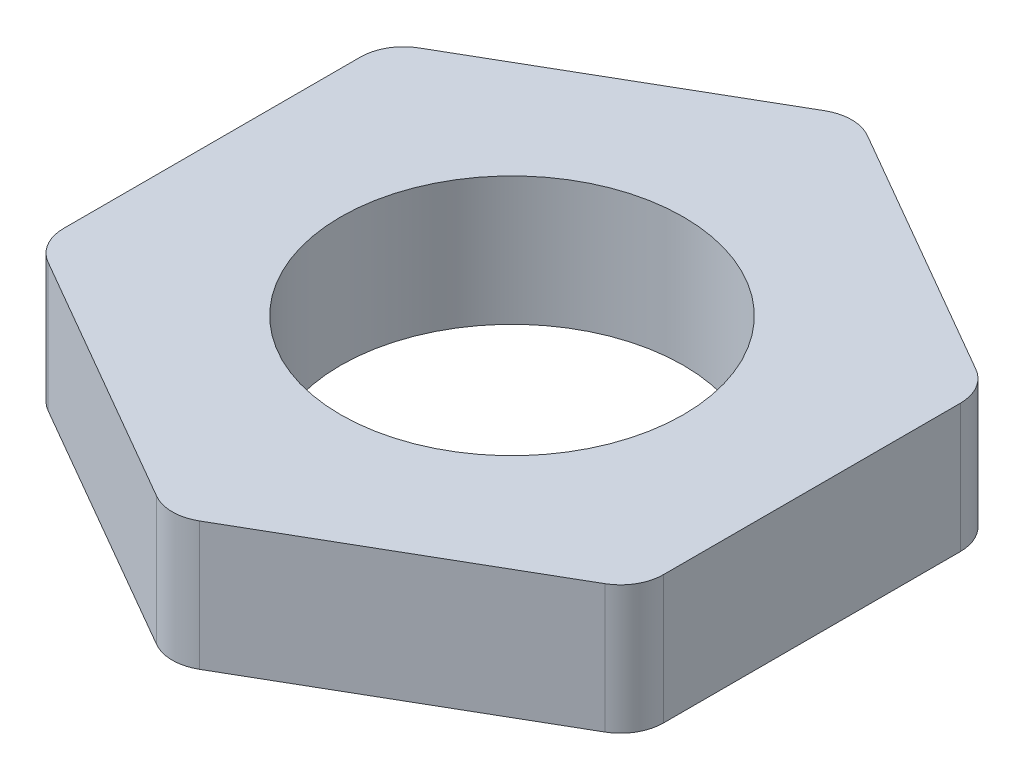
ISO-10303-21;
HEADER;
FILE_DESCRIPTION(('STEP AP214'),'2;1');
FILE_NAME('part.step','',(''),(''),'','','');
FILE_SCHEMA(('AUTOMOTIVE_DESIGN { 1 0 10303 214 1 1 1 1 }'));
ENDSEC;
DATA;
#1=APPLICATION_CONTEXT('core data for automotive mechanical design processes');
#2=APPLICATION_PROTOCOL_DEFINITION('international standard','automotive_design',2000,#1);
#3=PRODUCT_CONTEXT('',#1,'mechanical');
#4=PRODUCT('Part','Part','',(#3));
#5=PRODUCT_RELATED_PRODUCT_CATEGORY('part','',(#4));
#6=PRODUCT_DEFINITION_FORMATION('','',#4);
#7=PRODUCT_DEFINITION_CONTEXT('part definition',#1,'design');
#8=PRODUCT_DEFINITION('design','',#6,#7);
#9=PRODUCT_DEFINITION_SHAPE('','',#8);
#10=(LENGTH_UNIT() NAMED_UNIT(*) SI_UNIT(.MILLI.,.METRE.));
#11=(NAMED_UNIT(*) PLANE_ANGLE_UNIT() SI_UNIT($,.RADIAN.));
#12=(NAMED_UNIT(*) SI_UNIT($,.STERADIAN.) SOLID_ANGLE_UNIT());
#13=UNCERTAINTY_MEASURE_WITH_UNIT(LENGTH_MEASURE(1.E-05),#10,'distance_accuracy_value','');
#14=(GEOMETRIC_REPRESENTATION_CONTEXT(3) GLOBAL_UNCERTAINTY_ASSIGNED_CONTEXT((#13)) GLOBAL_UNIT_ASSIGNED_CONTEXT((#10,
#11,#12)) REPRESENTATION_CONTEXT('',''));
#15=CARTESIAN_POINT('',(0.,0.,0.));
#16=DIRECTION('',(0.,0.,1.));
#17=DIRECTION('',(1.,0.,0.));
#18=AXIS2_PLACEMENT_3D('',#15,#16,#17);
#19=CARTESIAN_POINT('',(7.,3.,-4.04145188432738));
#20=DIRECTION('',(-0.5,0.,0.866025403784439));
#21=DIRECTION('',(0.866025403784439,0.,0.5));
#22=AXIS2_PLACEMENT_3D('',#19,#20,#21);
#23=PLANE('',#22);
#24=DIRECTION('',(-0.866025403784439,0.,-0.5));
#25=VECTOR('',#24,1.);
#26=CARTESIAN_POINT('',(7.,0.,-4.04145188432738));
#27=LINE('',#26,#25);
#28=CARTESIAN_POINT('',(6.5,0.,-4.3301270189222));
#29=VERTEX_POINT('',#28);
#30=CARTESIAN_POINT('',(0.500000000000001,0.,-7.79422863405995));
#31=VERTEX_POINT('',#30);
#32=EDGE_CURVE('E223',#29,#31,#27,.T.);
#33=ORIENTED_EDGE('',*,*,#32,.T.);
#34=DIRECTION('',(0.,-1.,0.));
#35=VECTOR('',#34,1.);
#36=CARTESIAN_POINT('',(0.500000000000001,3.,-7.79422863405995));
#37=LINE('',#36,#35);
#38=CARTESIAN_POINT('',(0.500000000000001,3.,-7.79422863405995));
#39=VERTEX_POINT('',#38);
#40=EDGE_CURVE('E203',#31,#39,#37,.F.);
#41=ORIENTED_EDGE('',*,*,#40,.T.);
#42=DIRECTION('',(-0.866025403784439,0.,-0.5));
#43=VECTOR('',#42,1.);
#44=CARTESIAN_POINT('',(7.,3.,-4.04145188432738));
#45=LINE('',#44,#43);
#46=CARTESIAN_POINT('',(6.5,3.,-4.3301270189222));
#47=VERTEX_POINT('',#46);
#48=EDGE_CURVE('E169',#47,#39,#45,.T.);
#49=ORIENTED_EDGE('',*,*,#48,.F.);
#50=DIRECTION('',(0.,-1.,0.));
#51=VECTOR('',#50,1.);
#52=CARTESIAN_POINT('',(6.5,3.,-4.3301270189222));
#53=LINE('',#52,#51);
#54=EDGE_CURVE('E196',#47,#29,#53,.T.);
#55=ORIENTED_EDGE('',*,*,#54,.T.);
#56=EDGE_LOOP('',(#33,#41,#49,#55));
#57=FACE_BOUND('',#56,.T.);
#58=ADVANCED_FACE('F41',(#57),#23,.F.);
#59=CARTESIAN_POINT('',(0.,3.,-8.08290376865476));
#60=DIRECTION('',(0.5,0.,0.866025403784439));
#61=DIRECTION('',(0.866025403784439,0.,-0.5));
#62=AXIS2_PLACEMENT_3D('',#59,#60,#61);
#63=PLANE('',#62);
#64=DIRECTION('',(-0.866025403784439,0.,0.5));
#65=VECTOR('',#64,1.);
#66=CARTESIAN_POINT('',(0.,0.,-8.08290376865476));
#67=LINE('',#66,#65);
#68=CARTESIAN_POINT('',(-0.499999999999999,0.,-7.79422863405995));
#69=VERTEX_POINT('',#68);
#70=CARTESIAN_POINT('',(-6.5,0.,-4.3301270189222));
#71=VERTEX_POINT('',#70);
#72=EDGE_CURVE('E162',#69,#71,#67,.T.);
#73=ORIENTED_EDGE('',*,*,#72,.T.);
#74=DIRECTION('',(0.,-1.,0.));
#75=VECTOR('',#74,1.);
#76=CARTESIAN_POINT('',(-6.5,3.,-4.3301270189222));
#77=LINE('',#76,#75);
#78=CARTESIAN_POINT('',(-6.5,3.,-4.3301270189222));
#79=VERTEX_POINT('',#78);
#80=EDGE_CURVE('E198',#71,#79,#77,.F.);
#81=ORIENTED_EDGE('',*,*,#80,.T.);
#82=DIRECTION('',(-0.866025403784439,0.,0.5));
#83=VECTOR('',#82,1.);
#84=CARTESIAN_POINT('',(0.,3.,-8.08290376865476));
#85=LINE('',#84,#83);
#86=CARTESIAN_POINT('',(-0.499999999999999,3.,-7.79422863405995));
#87=VERTEX_POINT('',#86);
#88=EDGE_CURVE('E245',#87,#79,#85,.T.);
#89=ORIENTED_EDGE('',*,*,#88,.F.);
#90=DIRECTION('',(0.,-1.,0.));
#91=VECTOR('',#90,1.);
#92=CARTESIAN_POINT('',(-0.499999999999999,3.,-7.79422863405995));
#93=LINE('',#92,#91);
#94=EDGE_CURVE('E193',#87,#69,#93,.T.);
#95=ORIENTED_EDGE('',*,*,#94,.T.);
#96=EDGE_LOOP('',(#73,#81,#89,#95));
#97=FACE_BOUND('',#96,.T.);
#98=ADVANCED_FACE('F235',(#97),#63,.F.);
#99=CARTESIAN_POINT('',(-7.,3.,-4.04145188432738));
#100=DIRECTION('',(1.,0.,0.));
#101=DIRECTION('',(0.,0.,-1.));
#102=AXIS2_PLACEMENT_3D('',#99,#100,#101);
#103=PLANE('',#102);
#104=DIRECTION('',(0.,0.,1.));
#105=VECTOR('',#104,1.);
#106=CARTESIAN_POINT('',(-7.,0.,-4.04145188432738));
#107=LINE('',#106,#105);
#108=CARTESIAN_POINT('',(-7.,0.,-3.46410161513776));
#109=VERTEX_POINT('',#108);
#110=CARTESIAN_POINT('',(-7.,0.,3.46410161513775));
#111=VERTEX_POINT('',#110);
#112=EDGE_CURVE('E158',#109,#111,#107,.T.);
#113=ORIENTED_EDGE('',*,*,#112,.T.);
#114=DIRECTION('',(0.,-1.,0.));
#115=VECTOR('',#114,1.);
#116=CARTESIAN_POINT('',(-7.,3.,3.46410161513775));
#117=LINE('',#116,#115);
#118=CARTESIAN_POINT('',(-7.,3.,3.46410161513775));
#119=VERTEX_POINT('',#118);
#120=EDGE_CURVE('E137',#111,#119,#117,.F.);
#121=ORIENTED_EDGE('',*,*,#120,.T.);
#122=DIRECTION('',(0.,0.,1.));
#123=VECTOR('',#122,1.);
#124=CARTESIAN_POINT('',(-7.,3.,-4.04145188432738));
#125=LINE('',#124,#123);
#126=CARTESIAN_POINT('',(-7.,3.,-3.46410161513776));
#127=VERTEX_POINT('',#126);
#128=EDGE_CURVE('E242',#127,#119,#125,.T.);
#129=ORIENTED_EDGE('',*,*,#128,.F.);
#130=DIRECTION('',(0.,-1.,0.));
#131=VECTOR('',#130,1.);
#132=CARTESIAN_POINT('',(-7.,3.,-3.46410161513776));
#133=LINE('',#132,#131);
#134=EDGE_CURVE('E143',#127,#109,#133,.T.);
#135=ORIENTED_EDGE('',*,*,#134,.T.);
#136=EDGE_LOOP('',(#113,#121,#129,#135));
#137=FACE_BOUND('',#136,.T.);
#138=ADVANCED_FACE('F247',(#137),#103,.F.);
#139=CARTESIAN_POINT('',(-7.,3.,4.04145188432738));
#140=DIRECTION('',(0.5,0.,-0.866025403784439));
#141=DIRECTION('',(-0.866025403784439,0.,-0.5));
#142=AXIS2_PLACEMENT_3D('',#139,#140,#141);
#143=PLANE('',#142);
#144=DIRECTION('',(0.866025403784438,0.,0.5));
#145=VECTOR('',#144,1.);
#146=CARTESIAN_POINT('',(-7.,3.,4.04145188432738));
#147=LINE('',#146,#145);
#148=CARTESIAN_POINT('',(-6.5,3.,4.33012701892219));
#149=VERTEX_POINT('',#148);
#150=CARTESIAN_POINT('',(-0.500000000000004,3.,7.79422863405995));
#151=VERTEX_POINT('',#150);
#152=EDGE_CURVE('E151',#149,#151,#147,.T.);
#153=ORIENTED_EDGE('',*,*,#152,.F.);
#154=DIRECTION('',(0.,-1.,0.));
#155=VECTOR('',#154,1.);
#156=CARTESIAN_POINT('',(-6.5,3.,4.33012701892219));
#157=LINE('',#156,#155);
#158=CARTESIAN_POINT('',(-6.5,0.,4.33012701892219));
#159=VERTEX_POINT('',#158);
#160=EDGE_CURVE('E131',#149,#159,#157,.T.);
#161=ORIENTED_EDGE('',*,*,#160,.T.);
#162=DIRECTION('',(0.866025403784438,0.,0.5));
#163=VECTOR('',#162,1.);
#164=CARTESIAN_POINT('',(-7.,0.,4.04145188432738));
#165=LINE('',#164,#163);
#166=CARTESIAN_POINT('',(-0.500000000000004,0.,7.79422863405995));
#167=VERTEX_POINT('',#166);
#168=EDGE_CURVE('E146',#159,#167,#165,.T.);
#169=ORIENTED_EDGE('',*,*,#168,.T.);
#170=DIRECTION('',(0.,-1.,0.));
#171=VECTOR('',#170,1.);
#172=CARTESIAN_POINT('',(-0.500000000000002,3.,7.79422863405995));
#173=LINE('',#172,#171);
#174=EDGE_CURVE('E153',#167,#151,#173,.F.);
#175=ORIENTED_EDGE('',*,*,#174,.T.);
#176=EDGE_LOOP('',(#153,#161,#169,#175));
#177=FACE_BOUND('',#176,.T.);
#178=ADVANCED_FACE('F150',(#177),#143,.F.);
#179=CARTESIAN_POINT('',(0.,3.,8.08290376865476));
#180=DIRECTION('',(-0.5,0.,-0.866025403784439));
#181=DIRECTION('',(-0.866025403784439,0.,0.5));
#182=AXIS2_PLACEMENT_3D('',#179,#180,#181);
#183=PLANE('',#182);
#184=DIRECTION('',(0.866025403784439,0.,-0.5));
#185=VECTOR('',#184,1.);
#186=CARTESIAN_POINT('',(0.,0.,8.08290376865476));
#187=LINE('',#186,#185);
#188=CARTESIAN_POINT('',(0.499999999999998,0.,7.79422863405995));
#189=VERTEX_POINT('',#188);
#190=CARTESIAN_POINT('',(6.5,0.,4.33012701892219));
#191=VERTEX_POINT('',#190);
#192=EDGE_CURVE('E160',#189,#191,#187,.T.);
#193=ORIENTED_EDGE('',*,*,#192,.T.);
#194=DIRECTION('',(0.,-1.,0.));
#195=VECTOR('',#194,1.);
#196=CARTESIAN_POINT('',(6.5,3.,4.3301270189222));
#197=LINE('',#196,#195);
#198=CARTESIAN_POINT('',(6.5,3.,4.33012701892219));
#199=VERTEX_POINT('',#198);
#200=EDGE_CURVE('E11',#191,#199,#197,.F.);
#201=ORIENTED_EDGE('',*,*,#200,.T.);
#202=DIRECTION('',(0.866025403784439,0.,-0.5));
#203=VECTOR('',#202,1.);
#204=CARTESIAN_POINT('',(0.,3.,8.08290376865476));
#205=LINE('',#204,#203);
#206=CARTESIAN_POINT('',(0.499999999999998,3.,7.79422863405995));
#207=VERTEX_POINT('',#206);
#208=EDGE_CURVE('E215',#207,#199,#205,.T.);
#209=ORIENTED_EDGE('',*,*,#208,.F.);
#210=DIRECTION('',(0.,-1.,0.));
#211=VECTOR('',#210,1.);
#212=CARTESIAN_POINT('',(0.499999999999998,3.,7.79422863405995));
#213=LINE('',#212,#211);
#214=EDGE_CURVE('E47',#207,#189,#213,.T.);
#215=ORIENTED_EDGE('',*,*,#214,.T.);
#216=EDGE_LOOP('',(#193,#201,#209,#215));
#217=FACE_BOUND('',#216,.T.);
#218=ADVANCED_FACE('F209',(#217),#183,.F.);
#219=CARTESIAN_POINT('',(7.,3.,4.04145188432738));
#220=DIRECTION('',(-1.,0.,0.));
#221=DIRECTION('',(0.,0.,1.));
#222=AXIS2_PLACEMENT_3D('',#219,#220,#221);
#223=PLANE('',#222);
#224=DIRECTION('',(0.,0.,-1.));
#225=VECTOR('',#224,1.);
#226=CARTESIAN_POINT('',(7.,0.,4.04145188432738));
#227=LINE('',#226,#225);
#228=CARTESIAN_POINT('',(7.,0.,3.46410161513776));
#229=VERTEX_POINT('',#228);
#230=CARTESIAN_POINT('',(7.,0.,-3.46410161513776));
#231=VERTEX_POINT('',#230);
#232=EDGE_CURVE('E161',#229,#231,#227,.T.);
#233=ORIENTED_EDGE('',*,*,#232,.T.);
#234=DIRECTION('',(0.,-1.,0.));
#235=VECTOR('',#234,1.);
#236=CARTESIAN_POINT('',(7.,3.,-3.46410161513776));
#237=LINE('',#236,#235);
#238=CARTESIAN_POINT('',(7.,3.,-3.46410161513776));
#239=VERTEX_POINT('',#238);
#240=EDGE_CURVE('E57',#231,#239,#237,.F.);
#241=ORIENTED_EDGE('',*,*,#240,.T.);
#242=DIRECTION('',(0.,0.,-1.));
#243=VECTOR('',#242,1.);
#244=CARTESIAN_POINT('',(7.,3.,4.04145188432738));
#245=LINE('',#244,#243);
#246=CARTESIAN_POINT('',(7.,3.,3.46410161513776));
#247=VERTEX_POINT('',#246);
#248=EDGE_CURVE('E166',#247,#239,#245,.T.);
#249=ORIENTED_EDGE('',*,*,#248,.F.);
#250=DIRECTION('',(0.,-1.,0.));
#251=VECTOR('',#250,1.);
#252=CARTESIAN_POINT('',(7.,3.,3.46410161513776));
#253=LINE('',#252,#251);
#254=EDGE_CURVE('E201',#247,#229,#253,.T.);
#255=ORIENTED_EDGE('',*,*,#254,.T.);
#256=EDGE_LOOP('',(#233,#241,#249,#255));
#257=FACE_BOUND('',#256,.T.);
#258=ADVANCED_FACE('F218',(#257),#223,.F.);
#259=CARTESIAN_POINT('',(0.,3.,0.));
#260=DIRECTION('',(0.,1.,0.));
#261=DIRECTION('',(0.,0.,1.));
#262=AXIS2_PLACEMENT_3D('',#259,#260,#261);
#263=PLANE('',#262);
#264=CARTESIAN_POINT('',(0.,3.,0.));
#265=DIRECTION('',(0.,1.,0.));
#266=DIRECTION('',(0.,0.,1.));
#267=AXIS2_PLACEMENT_3D('',#264,#265,#266);
#268=CIRCLE('',#267,4.);
#269=CARTESIAN_POINT('',(0.,3.,4.));
#270=VERTEX_POINT('',#269);
#271=EDGE_CURVE('E252',#270,#270,#268,.T.);
#272=ORIENTED_EDGE('',*,*,#271,.F.);
#273=EDGE_LOOP('',(#272));
#274=FACE_BOUND('',#273,.T.);
#275=ORIENTED_EDGE('',*,*,#128,.T.);
#276=CARTESIAN_POINT('',(-6.,3.,3.46410161513775));
#277=DIRECTION('',(0.,1.,0.));
#278=DIRECTION('',(0.,0.,1.));
#279=AXIS2_PLACEMENT_3D('',#276,#277,#278);
#280=CIRCLE('',#279,1.);
#281=EDGE_CURVE('E192',#119,#149,#280,.T.);
#282=ORIENTED_EDGE('',*,*,#281,.T.);
#283=ORIENTED_EDGE('',*,*,#152,.T.);
#284=CARTESIAN_POINT('',(0.,3.,6.92820323027551));
#285=DIRECTION('',(0.,1.,0.));
#286=DIRECTION('',(0.,0.,1.));
#287=AXIS2_PLACEMENT_3D('',#284,#285,#286);
#288=CIRCLE('',#287,1.);
#289=EDGE_CURVE('E185',#151,#207,#288,.T.);
#290=ORIENTED_EDGE('',*,*,#289,.T.);
#291=ORIENTED_EDGE('',*,*,#208,.T.);
#292=CARTESIAN_POINT('',(6.,3.,3.46410161513776));
#293=DIRECTION('',(0.,1.,0.));
#294=DIRECTION('',(0.,0.,1.));
#295=AXIS2_PLACEMENT_3D('',#292,#293,#294);
#296=CIRCLE('',#295,1.);
#297=EDGE_CURVE('E62',#199,#247,#296,.T.);
#298=ORIENTED_EDGE('',*,*,#297,.T.);
#299=ORIENTED_EDGE('',*,*,#248,.T.);
#300=CARTESIAN_POINT('',(6.,3.,-3.46410161513776));
#301=DIRECTION('',(0.,1.,0.));
#302=DIRECTION('',(0.,0.,1.));
#303=AXIS2_PLACEMENT_3D('',#300,#301,#302);
#304=CIRCLE('',#303,1.);
#305=EDGE_CURVE('E183',#239,#47,#304,.T.);
#306=ORIENTED_EDGE('',*,*,#305,.T.);
#307=ORIENTED_EDGE('',*,*,#48,.T.);
#308=CARTESIAN_POINT('',(0.,3.,-6.92820323027551));
#309=DIRECTION('',(0.,1.,0.));
#310=DIRECTION('',(0.,0.,1.));
#311=AXIS2_PLACEMENT_3D('',#308,#309,#310);
#312=CIRCLE('',#311,1.);
#313=EDGE_CURVE('E189',#39,#87,#312,.T.);
#314=ORIENTED_EDGE('',*,*,#313,.T.);
#315=ORIENTED_EDGE('',*,*,#88,.T.);
#316=CARTESIAN_POINT('',(-6.,3.,-3.46410161513776));
#317=DIRECTION('',(0.,1.,0.));
#318=DIRECTION('',(0.,0.,1.));
#319=AXIS2_PLACEMENT_3D('',#316,#317,#318);
#320=CIRCLE('',#319,1.);
#321=EDGE_CURVE('E190',#79,#127,#320,.T.);
#322=ORIENTED_EDGE('',*,*,#321,.T.);
#323=EDGE_LOOP('',(#275,#282,#283,#290,#291,#298,#299,#306,#307,#314,#315,#322));
#324=FACE_BOUND('',#323,.T.);
#325=ADVANCED_FACE('F244',(#274,#324),#263,.T.);
#326=CARTESIAN_POINT('',(0.,0.,0.));
#327=DIRECTION('',(0.,1.,0.));
#328=DIRECTION('',(0.,0.,1.));
#329=AXIS2_PLACEMENT_3D('',#326,#327,#328);
#330=PLANE('',#329);
#331=CARTESIAN_POINT('',(0.,0.,0.));
#332=DIRECTION('',(0.,1.,0.));
#333=DIRECTION('',(0.,0.,1.));
#334=AXIS2_PLACEMENT_3D('',#331,#332,#333);
#335=CIRCLE('',#334,4.);
#336=CARTESIAN_POINT('',(0.,0.,4.));
#337=VERTEX_POINT('',#336);
#338=EDGE_CURVE('E229',#337,#337,#335,.T.);
#339=ORIENTED_EDGE('',*,*,#338,.T.);
#340=EDGE_LOOP('',(#339));
#341=FACE_BOUND('',#340,.T.);
#342=ORIENTED_EDGE('',*,*,#168,.F.);
#343=CARTESIAN_POINT('',(-6.,0.,3.46410161513775));
#344=DIRECTION('',(0.,1.,0.));
#345=DIRECTION('',(0.,0.,1.));
#346=AXIS2_PLACEMENT_3D('',#343,#344,#345);
#347=CIRCLE('',#346,1.);
#348=EDGE_CURVE('E133',#159,#111,#347,.F.);
#349=ORIENTED_EDGE('',*,*,#348,.T.);
#350=ORIENTED_EDGE('',*,*,#112,.F.);
#351=CARTESIAN_POINT('',(-6.,0.,-3.46410161513776));
#352=DIRECTION('',(0.,1.,0.));
#353=DIRECTION('',(0.,0.,1.));
#354=AXIS2_PLACEMENT_3D('',#351,#352,#353);
#355=CIRCLE('',#354,1.);
#356=EDGE_CURVE('E142',#109,#71,#355,.F.);
#357=ORIENTED_EDGE('',*,*,#356,.T.);
#358=ORIENTED_EDGE('',*,*,#72,.F.);
#359=CARTESIAN_POINT('',(0.,0.,-6.92820323027551));
#360=DIRECTION('',(0.,1.,0.));
#361=DIRECTION('',(0.,0.,1.));
#362=AXIS2_PLACEMENT_3D('',#359,#360,#361);
#363=CIRCLE('',#362,1.);
#364=EDGE_CURVE('E177',#69,#31,#363,.F.);
#365=ORIENTED_EDGE('',*,*,#364,.T.);
#366=ORIENTED_EDGE('',*,*,#32,.F.);
#367=CARTESIAN_POINT('',(6.,0.,-3.46410161513776));
#368=DIRECTION('',(0.,1.,0.));
#369=DIRECTION('',(0.,0.,1.));
#370=AXIS2_PLACEMENT_3D('',#367,#368,#369);
#371=CIRCLE('',#370,1.);
#372=EDGE_CURVE('E175',#29,#231,#371,.F.);
#373=ORIENTED_EDGE('',*,*,#372,.T.);
#374=ORIENTED_EDGE('',*,*,#232,.F.);
#375=CARTESIAN_POINT('',(6.,0.,3.46410161513776));
#376=DIRECTION('',(0.,1.,0.));
#377=DIRECTION('',(0.,0.,1.));
#378=AXIS2_PLACEMENT_3D('',#375,#376,#377);
#379=CIRCLE('',#378,1.);
#380=EDGE_CURVE('E174',#229,#191,#379,.F.);
#381=ORIENTED_EDGE('',*,*,#380,.T.);
#382=ORIENTED_EDGE('',*,*,#192,.F.);
#383=CARTESIAN_POINT('',(0.,0.,6.92820323027551));
#384=DIRECTION('',(0.,1.,0.));
#385=DIRECTION('',(0.,0.,1.));
#386=AXIS2_PLACEMENT_3D('',#383,#384,#385);
#387=CIRCLE('',#386,1.);
#388=EDGE_CURVE('E155',#189,#167,#387,.F.);
#389=ORIENTED_EDGE('',*,*,#388,.T.);
#390=EDGE_LOOP('',(#342,#349,#350,#357,#358,#365,#366,#373,#374,#381,#382,#389));
#391=FACE_BOUND('',#390,.T.);
#392=ADVANCED_FACE('F154',(#341,#391),#330,.F.);
#393=CARTESIAN_POINT('',(0.,0.,0.));
#394=DIRECTION('',(0.,1.,0.));
#395=DIRECTION('',(0.,0.,1.));
#396=AXIS2_PLACEMENT_3D('',#393,#394,#395);
#397=CYLINDRICAL_SURFACE('',#396,4.);
#398=ORIENTED_EDGE('',*,*,#338,.F.);
#399=EDGE_LOOP('',(#398));
#400=FACE_BOUND('',#399,.T.);
#401=ORIENTED_EDGE('',*,*,#271,.T.);
#402=EDGE_LOOP('',(#401));
#403=FACE_BOUND('',#402,.T.);
#404=ADVANCED_FACE('F259',(#400,#403),#397,.F.);
#405=CARTESIAN_POINT('',(-6.,3.,3.46410161513775));
#406=DIRECTION('',(0.,-1.,0.));
#407=DIRECTION('',(0.,0.,-1.));
#408=AXIS2_PLACEMENT_3D('',#405,#406,#407);
#409=CYLINDRICAL_SURFACE('',#408,1.);
#410=ORIENTED_EDGE('',*,*,#281,.F.);
#411=ORIENTED_EDGE('',*,*,#120,.F.);
#412=ORIENTED_EDGE('',*,*,#348,.F.);
#413=ORIENTED_EDGE('',*,*,#160,.F.);
#414=EDGE_LOOP('',(#410,#411,#412,#413));
#415=FACE_BOUND('',#414,.T.);
#416=ADVANCED_FACE('F135',(#415),#409,.T.);
#417=CARTESIAN_POINT('',(-6.,3.,-3.46410161513776));
#418=DIRECTION('',(0.,-1.,0.));
#419=DIRECTION('',(0.,0.,-1.));
#420=AXIS2_PLACEMENT_3D('',#417,#418,#419);
#421=CYLINDRICAL_SURFACE('',#420,1.);
#422=ORIENTED_EDGE('',*,*,#321,.F.);
#423=ORIENTED_EDGE('',*,*,#80,.F.);
#424=ORIENTED_EDGE('',*,*,#356,.F.);
#425=ORIENTED_EDGE('',*,*,#134,.F.);
#426=EDGE_LOOP('',(#422,#423,#424,#425));
#427=FACE_BOUND('',#426,.T.);
#428=ADVANCED_FACE('F236',(#427),#421,.T.);
#429=CARTESIAN_POINT('',(0.,3.,-6.92820323027551));
#430=DIRECTION('',(0.,-1.,0.));
#431=DIRECTION('',(0.,0.,-1.));
#432=AXIS2_PLACEMENT_3D('',#429,#430,#431);
#433=CYLINDRICAL_SURFACE('',#432,1.);
#434=ORIENTED_EDGE('',*,*,#313,.F.);
#435=ORIENTED_EDGE('',*,*,#40,.F.);
#436=ORIENTED_EDGE('',*,*,#364,.F.);
#437=ORIENTED_EDGE('',*,*,#94,.F.);
#438=EDGE_LOOP('',(#434,#435,#436,#437));
#439=FACE_BOUND('',#438,.T.);
#440=ADVANCED_FACE('F287',(#439),#433,.T.);
#441=CARTESIAN_POINT('',(6.,3.,-3.46410161513776));
#442=DIRECTION('',(0.,-1.,0.));
#443=DIRECTION('',(0.,0.,-1.));
#444=AXIS2_PLACEMENT_3D('',#441,#442,#443);
#445=CYLINDRICAL_SURFACE('',#444,1.);
#446=ORIENTED_EDGE('',*,*,#305,.F.);
#447=ORIENTED_EDGE('',*,*,#240,.F.);
#448=ORIENTED_EDGE('',*,*,#372,.F.);
#449=ORIENTED_EDGE('',*,*,#54,.F.);
#450=EDGE_LOOP('',(#446,#447,#448,#449));
#451=FACE_BOUND('',#450,.T.);
#452=ADVANCED_FACE('F289',(#451),#445,.T.);
#453=CARTESIAN_POINT('',(6.,3.,3.46410161513776));
#454=DIRECTION('',(0.,-1.,0.));
#455=DIRECTION('',(0.,0.,-1.));
#456=AXIS2_PLACEMENT_3D('',#453,#454,#455);
#457=CYLINDRICAL_SURFACE('',#456,1.);
#458=ORIENTED_EDGE('',*,*,#297,.F.);
#459=ORIENTED_EDGE('',*,*,#200,.F.);
#460=ORIENTED_EDGE('',*,*,#380,.F.);
#461=ORIENTED_EDGE('',*,*,#254,.F.);
#462=EDGE_LOOP('',(#458,#459,#460,#461));
#463=FACE_BOUND('',#462,.T.);
#464=ADVANCED_FACE('F217',(#463),#457,.T.);
#465=CARTESIAN_POINT('',(0.,3.,6.92820323027551));
#466=DIRECTION('',(0.,-1.,0.));
#467=DIRECTION('',(0.,0.,-1.));
#468=AXIS2_PLACEMENT_3D('',#465,#466,#467);
#469=CYLINDRICAL_SURFACE('',#468,1.);
#470=ORIENTED_EDGE('',*,*,#289,.F.);
#471=ORIENTED_EDGE('',*,*,#174,.F.);
#472=ORIENTED_EDGE('',*,*,#388,.F.);
#473=ORIENTED_EDGE('',*,*,#214,.F.);
#474=EDGE_LOOP('',(#470,#471,#472,#473));
#475=FACE_BOUND('',#474,.T.);
#476=ADVANCED_FACE('F43',(#475),#469,.T.);
#477=CLOSED_SHELL('',(#58,#98,#138,#178,#218,#258,#325,#392,#404,#416,#428,#440,#452,#464,#476));
#478=MANIFOLD_SOLID_BREP('B2',#477);
#479=ADVANCED_BREP_SHAPE_REPRESENTATION('',(#18,#478),#14);
#480=SHAPE_DEFINITION_REPRESENTATION(#9,#479);
ENDSEC;
END-ISO-10303-21;
